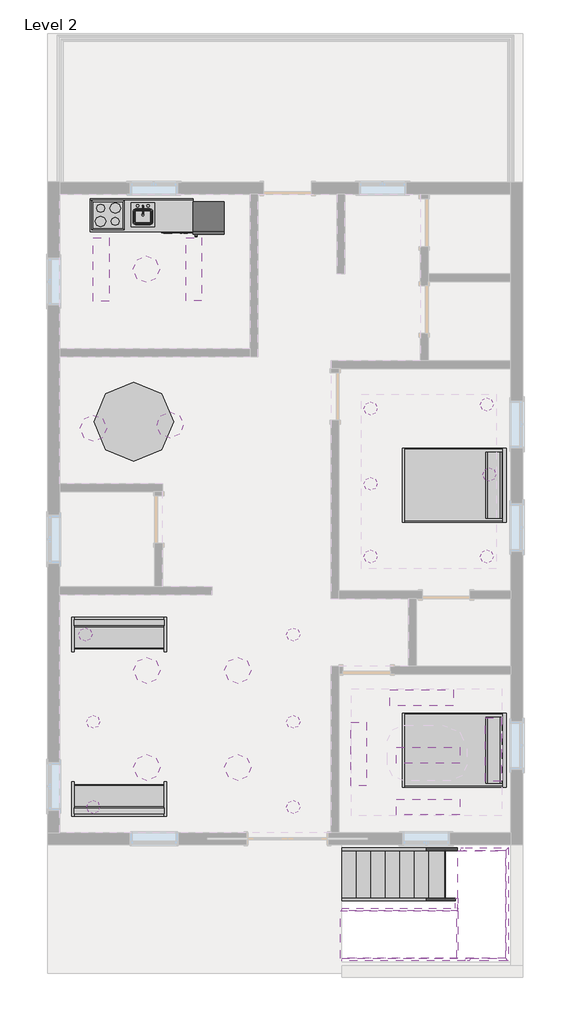
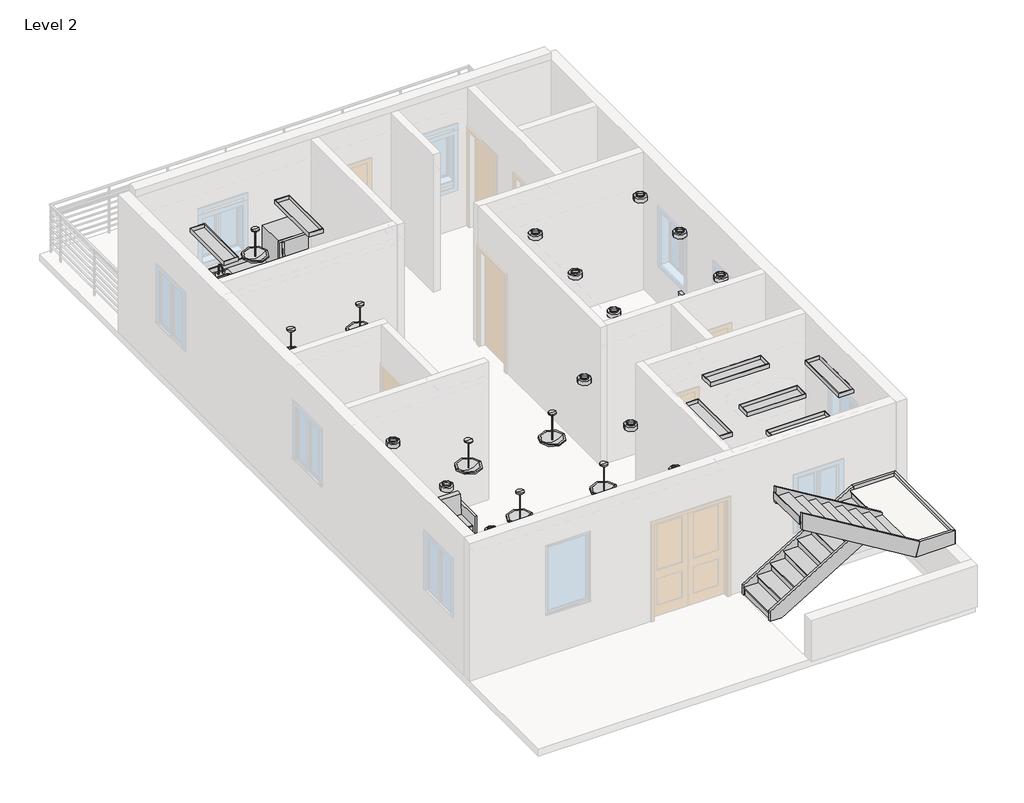
# One storey, part 3 of 3: 26 light fixtures, 8 members, 6 furniture elements, 4 proxies, 2 stair flights, 1 flow terminal, 1 slab.
"""IFC4 building model written with IfcOpenShell, lengths in millimetres."""

from ifc_helpers import new_model, si_unit, frame, origin, place, context, project, spatial, polyline, outline, extrude, faceted_brep, transform, mapped, element, save
from components import proxy_a6faaae8, proxy_45b28599, kitchenette_medium_kitchenette_medium_844211aa, proxy_c523a7b7, flow_terminal_871c2e40, furniture_096e7f55, furniture_c6510c7c, m_sofa_1830mm_f9e8a66b, furniture_bbcc68ce, ceiling_light_flat_round_60w_120v_0a96185f, ceiling_light_linear_box_1_x4_1_lamp_120v_8873ebfc, pendant_light_hemisphere_100w_120v_9c66a66f, non_monolithic_landing_dfce8634, stair_flight_5af034e0, stair_flight_d8780985

model = new_model("IFC4")

# Units and contexts
model_context = context("Model", 3, world=origin())
ifc_project = project(units=[si_unit("LENGTHUNIT", "METRE", prefix="MILLI")], contexts=[model_context])

# Site, building, storey
site = spatial("IfcSite", under=ifc_project)
building = spatial("IfcBuilding", under=site)
storey = spatial("IfcBuildingStorey", under=building, Name="Level 2", Elevation=3200.4)

# Proxies
placement = place(None, origin())
proxy_shape = proxy_a6faaae8(model_context)
element("IfcBuildingElementProxy", 1, Name="Cook Top-4 Unit2 : 22\" x 20\"", ObjectType="Cook Top-4 Unit2 : 22\" x 20\"", at=placement, inside=storey, context=model_context, shape_type="MappedRepresentation", body=[
    mapped(proxy_shape, transform((-8911.7572065, 13575.3206867, 3200.4), x_axis=(1.0, 0.0, 0.0), y_axis=(0.0, 1.0, 0.0), z_axis=(0.0, 0.0, 1.0))),
])
proxy_2_shape = proxy_45b28599(model_context)
element("IfcBuildingElementProxy", 2, Name="Dishwasher : 24\" x 24\" x 34\"", ObjectType="Dishwasher : 24\" x 24\" x 34\"", at=placement, inside=storey, context=model_context, shape_type="MappedRepresentation", body=[
    mapped(proxy_2_shape, transform((-7960.574675, 13283.4711219, 3200.4), x_axis=(1.0, 0.0, 0.0), y_axis=(0.0, 1.0, 0.0), z_axis=(0.0, 0.0, 1.0))),
])
kitchenette_medium_kitchenette_medium_shape = kitchenette_medium_kitchenette_medium_844211aa(model_context)
element("IfcBuildingElementProxy", 3, Name="Kitchenette - Medium : Kitchenette - Medium", ObjectType="Kitchenette - Medium : Kitchenette - Medium", at=placement, inside=storey, context=model_context, shape_type="MappedRepresentation", body=[
    mapped(kitchenette_medium_kitchenette_medium_shape, transform((-8587.5949114, 13880.1206867, 3200.4), x_axis=(1.0, 0.0, 0.0), y_axis=(0.0, 1.0, 0.0), z_axis=(0.0, 0.0, 1.0))),
])
proxy_3_shape = proxy_c523a7b7(model_context)
element("IfcBuildingElementProxy", 4, Name="Refrigerator : 24\" x 25\" LH", ObjectType="Refrigerator : 24\" x 25\" LH", at=placement, inside=storey, context=model_context, shape_type="MappedRepresentation", body=[
    mapped(proxy_3_shape, transform((-6975.0072065, 13529.6717152, 3200.4), x_axis=(1.0, 0.0, 0.0), y_axis=(0.0, 1.0, 0.0), z_axis=(0.0, 0.0, 1.0))),
])

# Flow terminal
flow_terminal_shape = flow_terminal_871c2e40(model_context)
element("IfcFlowTerminal", 5, ObjectType="Sink Kitchen-Island : 18\" x 18\"", at=placement, inside=storey, context=model_context, shape_type="MappedRepresentation", body=[
    mapped(flow_terminal_shape, transform((-8254.3464471, 13572.9752855, 3186.0), x_axis=(1.0, 0.0, 0.0), y_axis=(0.0, 1.0, 0.0), z_axis=(0.0, 0.0, 1.0))),
])

# Furniture
furniture_shape = furniture_096e7f55(model_context)
element("IfcFurniture", 6, ObjectType="Bed-Shaker : Double 56\" x 78\"", at=placement, inside=storey, context=model_context, shape_type="MappedRepresentation", body=[
    mapped(furniture_shape, transform((-1266.3572065, 8361.9706867, 3200.4), x_axis=(0.0, -1.0000000000000007, 0.0), y_axis=(1.0000000000000007, 0.0, 0.0), z_axis=(0.0, 0.0, 1.0))),
])
element("IfcFurniture", 7, ObjectType="Bed-Shaker : Double 56\" x 78\"", at=placement, inside=storey, context=model_context, shape_type="MappedRepresentation", body=[
    mapped(furniture_shape, transform((-1266.3572065, 3269.2706867, 3200.4), x_axis=(0.0, -1.0, 0.0), y_axis=(1.0, 0.0, 0.0), z_axis=(0.0, 0.0, 1.0))),
])
furniture_2_shape = furniture_c6510c7c(model_context)
element("IfcFurniture", 8, ObjectType="Counter Top w Sink Hole : 24\" Depth", at=placement, inside=storey, context=model_context, shape_type="MappedRepresentation", body=[
    mapped(furniture_2_shape, transform((-8054.1949114, 13880.1206867, 3186.0), x_axis=(1.0, 0.0, 0.0), y_axis=(0.0, 1.0, 0.0), z_axis=(0.0, 0.0, 1.0))),
])
m_sofa_1830mm_shape = m_sofa_1830mm_f9e8a66b(model_context)
element("IfcFurniture", 9, ObjectType="M_Sofa : 1830mm", at=placement, inside=storey, context=model_context, shape_type="MappedRepresentation", body=[
    mapped(m_sofa_1830mm_shape, transform((-8766.2276983, 5364.6665883, 3200.4), x_axis=(1.0, 0.0, 0.0), y_axis=(0.0, 1.0, 0.0), z_axis=(0.0, 0.0, 1.0))),
])
element("IfcFurniture", 10, ObjectType="M_Sofa : 1830mm", at=placement, inside=storey, context=model_context, shape_type="MappedRepresentation", body=[
    mapped(m_sofa_1830mm_shape, transform((-8625.4867147, 2494.674785, 3200.4), x_axis=(-1.0000000000000002, 0.0, 0.0), y_axis=(0.0, -1.0000000000000002, 0.0), z_axis=(0.0, 0.0, 1.0))),
])
furniture_3_shape = furniture_bbcc68ce(model_context)
element("IfcFurniture", 11, ObjectType="Table-Dining Round w Chairs : 60\" Diameter", at=placement, inside=storey, context=model_context, shape_type="MappedRepresentation", body=[
    mapped(furniture_3_shape, transform((-8517.0768878, 9782.3608189, 3200.4), x_axis=(1.0, 0.0, 0.0), y_axis=(0.0, 1.0, 0.0), z_axis=(0.0, 0.0, 1.0))),
])

# Light fixtures
ceiling_light_flat_round_60w_120v_shape = ceiling_light_flat_round_60w_120v_0a96185f(model_context)
element("IfcLightFixture", 12, ObjectType="Ceiling Light - Flat Round : 60W - 120V", at=placement, inside=storey, context=model_context, shape_type="MappedRepresentation", body=[
    mapped(ceiling_light_flat_round_60w_120v_shape, transform((-9343.5572065, 5510.8206867, 3403.6), x_axis=(1.0, 0.0, 0.0), y_axis=(0.0, 1.0, 0.0), z_axis=(0.0, 0.0, 1.0))),
])
element("IfcLightFixture", 13, ObjectType="Ceiling Light - Flat Round : 60W - 120V", at=placement, inside=storey, context=model_context, shape_type="MappedRepresentation", body=[
    mapped(ceiling_light_flat_round_60w_120v_shape, transform((-5345.2061474, 5507.5682565, 3403.6), x_axis=(1.0, 0.0, 0.0), y_axis=(0.0, 1.0, 0.0), z_axis=(0.0, 0.0, 1.0))),
])
element("IfcLightFixture", 14, ObjectType="Ceiling Light - Flat Round : 60W - 120V", at=placement, inside=storey, context=model_context, shape_type="MappedRepresentation", body=[
    mapped(ceiling_light_flat_round_60w_120v_shape, transform((-9193.3061474, 3831.1682565, 3403.6), x_axis=(1.0, 0.0, 0.0), y_axis=(0.0, 1.0, 0.0), z_axis=(0.0, 0.0, 1.0))),
])
element("IfcLightFixture", 15, ObjectType="Ceiling Light - Flat Round : 60W - 120V", at=placement, inside=storey, context=model_context, shape_type="MappedRepresentation", body=[
    mapped(ceiling_light_flat_round_60w_120v_shape, transform((-5345.2061474, 3831.1682565, 3403.6), x_axis=(1.0, 0.0, 0.0), y_axis=(0.0, 1.0, 0.0), z_axis=(0.0, 0.0, 1.0))),
])
element("IfcLightFixture", 16, ObjectType="Ceiling Light - Flat Round : 60W - 120V", at=placement, inside=storey, context=model_context, shape_type="MappedRepresentation", body=[
    mapped(ceiling_light_flat_round_60w_120v_shape, transform((-9193.3061474, 2192.8682565, 3403.6), x_axis=(1.0, 0.0, 0.0), y_axis=(0.0, 1.0, 0.0), z_axis=(0.0, 0.0, 1.0))),
])
element("IfcLightFixture", 17, ObjectType="Ceiling Light - Flat Round : 60W - 120V", at=placement, inside=storey, context=model_context, shape_type="MappedRepresentation", body=[
    mapped(ceiling_light_flat_round_60w_120v_shape, transform((-5345.2061474, 2192.8682565, 3403.6), x_axis=(1.0, 0.0, 0.0), y_axis=(0.0, 1.0, 0.0), z_axis=(0.0, 0.0, 1.0))),
])
element("IfcLightFixture", 18, ObjectType="Ceiling Light - Flat Round : 60W - 277V", at=placement, inside=storey, context=model_context, shape_type="MappedRepresentation", body=[
    mapped(ceiling_light_flat_round_60w_120v_shape, transform((-3860.0824155, 9852.6859166, 3454.4), x_axis=(1.0, 0.0, 0.0), y_axis=(0.0, 1.0, 0.0), z_axis=(0.0, 0.0, 1.0))),
])
element("IfcLightFixture", 19, ObjectType="Ceiling Light - Flat Round : 60W - 277V", at=placement, inside=storey, context=model_context, shape_type="MappedRepresentation", body=[
    mapped(ceiling_light_flat_round_60w_120v_shape, transform((-1624.8824155, 9928.8859166, 3454.4), x_axis=(1.0, 0.0, 0.0), y_axis=(0.0, 1.0, 0.0), z_axis=(0.0, 0.0, 1.0))),
])
element("IfcLightFixture", 20, ObjectType="Ceiling Light - Flat Round : 60W - 277V", at=placement, inside=storey, context=model_context, shape_type="MappedRepresentation", body=[
    mapped(ceiling_light_flat_round_60w_120v_shape, transform((-1574.0824155, 8582.6859166, 3454.4), x_axis=(1.0, 0.0, 0.0), y_axis=(0.0, 1.0, 0.0), z_axis=(0.0, 0.0, 1.0))),
])
element("IfcLightFixture", 21, ObjectType="Ceiling Light - Flat Round : 60W - 277V", at=placement, inside=storey, context=model_context, shape_type="MappedRepresentation", body=[
    mapped(ceiling_light_flat_round_60w_120v_shape, transform((-3860.0824155, 8404.8859166, 3454.4), x_axis=(1.0, 0.0, 0.0), y_axis=(0.0, 1.0, 0.0), z_axis=(0.0, 0.0, 1.0))),
])
element("IfcLightFixture", 22, ObjectType="Ceiling Light - Flat Round : 60W - 277V", at=placement, inside=storey, context=model_context, shape_type="MappedRepresentation", body=[
    mapped(ceiling_light_flat_round_60w_120v_shape, transform((-3860.0824155, 7007.8859166, 3454.4), x_axis=(1.0, 0.0, 0.0), y_axis=(0.0, 1.0, 0.0), z_axis=(0.0, 0.0, 1.0))),
])
element("IfcLightFixture", 23, ObjectType="Ceiling Light - Flat Round : 60W - 277V", at=placement, inside=storey, context=model_context, shape_type="MappedRepresentation", body=[
    mapped(ceiling_light_flat_round_60w_120v_shape, transform((-1624.8824155, 7007.8859166, 3454.4), x_axis=(1.0, 0.0, 0.0), y_axis=(0.0, 1.0, 0.0), z_axis=(0.0, 0.0, 1.0))),
])
ceiling_light_linear_box_1_x4_1_lamp_120v_shape = ceiling_light_linear_box_1_x4_1_lamp_120v_8873ebfc(model_context)
element("IfcLightFixture", 24, ObjectType="Ceiling Light - Linear Box : 1'x4'(1 Lamp) - 120V", at=placement, inside=storey, context=model_context, shape_type="MappedRepresentation", body=[
    mapped(ceiling_light_linear_box_1_x4_1_lamp_120v_shape, transform((-9038.7572065, 12521.2206867, 3403.6), x_axis=(0.0, 1.0000000000000002, 0.0), y_axis=(-1.0000000000000002, 0.0, 0.0), z_axis=(0.0, 0.0, 1.0))),
])
element("IfcLightFixture", 25, ObjectType="Ceiling Light - Linear Box : 1'x4'(1 Lamp) - 120V", at=placement, inside=storey, context=model_context, shape_type="MappedRepresentation", body=[
    mapped(ceiling_light_linear_box_1_x4_1_lamp_120v_shape, transform((-7259.0575781, 12529.2390316, 3403.6), x_axis=(0.0, -1.0000000000000007, 0.0), y_axis=(1.0000000000000007, 0.0, 0.0), z_axis=(0.0, 0.0, 1.0))),
])
element("IfcLightFixture", 26, ObjectType="Ceiling Light - Linear Box : 1'x4'(2 Lamp) - 120V", at=placement, inside=storey, context=model_context, shape_type="MappedRepresentation", body=[
    mapped(ceiling_light_linear_box_1_x4_1_lamp_120v_shape, transform((-2753.8070542, 3185.9258823, 3403.6), x_axis=(1.0, 0.0, 0.0), y_axis=(0.0, 1.0, 0.0), z_axis=(0.0, 0.0, 1.0))),
])
element("IfcLightFixture", 27, ObjectType="Ceiling Light - Linear Box : 1'x4'(2 Lamp) - 120V", at=placement, inside=storey, context=model_context, shape_type="MappedRepresentation", body=[
    mapped(ceiling_light_linear_box_1_x4_1_lamp_120v_shape, transform((-2880.8070542, 4290.8258823, 3441.6205268), x_axis=(1.0, 0.0, 0.0), y_axis=(0.0, 1.0, 0.0), z_axis=(0.0, 0.0, 1.0))),
])
element("IfcLightFixture", 28, ObjectType="Ceiling Light - Linear Box : 1'x4'(2 Lamp) - 120V", at=placement, inside=storey, context=model_context, shape_type="MappedRepresentation", body=[
    mapped(ceiling_light_linear_box_1_x4_1_lamp_120v_shape, transform((-2753.8070542, 2195.3258823, 3441.6205268), x_axis=(1.0, 0.0, 0.0), y_axis=(0.0, 1.0, 0.0), z_axis=(0.0, 0.0, 1.0))),
])
element("IfcLightFixture", 29, ObjectType="Ceiling Light - Linear Box : 1'x4'(2 Lamp) - 120V", at=placement, inside=storey, context=model_context, shape_type="MappedRepresentation", body=[
    mapped(ceiling_light_linear_box_1_x4_1_lamp_120v_shape, transform((-1496.5070542, 3300.2258823, 3441.6205268), x_axis=(0.0, 1.0000000000000002, 0.0), y_axis=(-1.0000000000000002, 0.0, 0.0), z_axis=(0.0, 0.0, 1.0))),
])
element("IfcLightFixture", 30, ObjectType="Ceiling Light - Linear Box : 1'x4'(2 Lamp) - 120V", at=placement, inside=storey, context=model_context, shape_type="MappedRepresentation", body=[
    mapped(ceiling_light_linear_box_1_x4_1_lamp_120v_shape, transform((-4087.3070542, 3211.3258823, 3441.6205268), x_axis=(0.0, 1.0000000000000002, 0.0), y_axis=(-1.0000000000000002, 0.0, 0.0), z_axis=(0.0, 0.0, 1.0))),
])
pendant_light_hemisphere_100w_120v_shape = pendant_light_hemisphere_100w_120v_9c66a66f(model_context)
element("IfcLightFixture", 31, ObjectType="Pendant Light - Hemisphere : 100W - 120V", at=placement, inside=storey, context=model_context, shape_type="MappedRepresentation", body=[
    mapped(pendant_light_hemisphere_100w_120v_shape, transform((-8164.6061474, 2954.8682565, 3403.6), x_axis=(1.0, 0.0, 0.0), y_axis=(0.0, 1.0, 0.0), z_axis=(0.0, 0.0, 1.0))),
])
element("IfcLightFixture", 32, ObjectType="Pendant Light - Hemisphere : 100W - 120V", at=placement, inside=storey, context=model_context, shape_type="MappedRepresentation", body=[
    mapped(pendant_light_hemisphere_100w_120v_shape, transform((-8164.6061474, 4821.7682565, 3403.6), x_axis=(1.0, 0.0, 0.0), y_axis=(0.0, 1.0, 0.0), z_axis=(0.0, 0.0, 1.0))),
])
element("IfcLightFixture", 33, ObjectType="Pendant Light - Hemisphere : 100W - 120V", at=placement, inside=storey, context=model_context, shape_type="MappedRepresentation", body=[
    mapped(pendant_light_hemisphere_100w_120v_shape, transform((-6412.0061474, 4821.7682565, 3403.6), x_axis=(1.0, 0.0, 0.0), y_axis=(0.0, 1.0, 0.0), z_axis=(0.0, 0.0, 1.0))),
])
element("IfcLightFixture", 34, ObjectType="Pendant Light - Hemisphere : 100W - 120V", at=placement, inside=storey, context=model_context, shape_type="MappedRepresentation", body=[
    mapped(pendant_light_hemisphere_100w_120v_shape, transform((-6412.0061474, 2954.8682565, 3403.6), x_axis=(1.0, 0.0, 0.0), y_axis=(0.0, 1.0, 0.0), z_axis=(0.0, 0.0, 1.0))),
])
element("IfcLightFixture", 35, ObjectType="Pendant Light - Hemisphere : 100W - 120V", at=placement, inside=storey, context=model_context, shape_type="MappedRepresentation", body=[
    mapped(pendant_light_hemisphere_100w_120v_shape, transform((-9191.1572065, 9473.2206867, 3403.6), x_axis=(1.0, 0.0, 0.0), y_axis=(0.0, 1.0, 0.0), z_axis=(0.0, 0.0, 1.0))),
])
element("IfcLightFixture", 36, ObjectType="Pendant Light - Hemisphere : 100W - 120V", at=placement, inside=storey, context=model_context, shape_type="MappedRepresentation", body=[
    mapped(pendant_light_hemisphere_100w_120v_shape, transform((-7715.9326808, 9533.782557, 3403.6), x_axis=(1.0, 0.0, 0.0), y_axis=(0.0, 1.0, 0.0), z_axis=(0.0, 0.0, 1.0))),
])
element("IfcLightFixture", 37, ObjectType="Pendant Light - Hemisphere : 100W - 120V", at=placement, inside=storey, context=model_context, shape_type="MappedRepresentation", body=[
    mapped(pendant_light_hemisphere_100w_120v_shape, transform((-8173.4575781, 12529.2390316, 3403.6), x_axis=(1.0, 0.0, 0.0), y_axis=(0.0, 1.0, 0.0), z_axis=(0.0, 0.0, 1.0))),
])

# Members
element("IfcMember", 38, ObjectType="Stringer - 2\" Width", at=placement, inside=storey, context=model_context, shape_type="SweptSolid", body=[
    extrude(outline(polyline([(3412.514512, -4412.1017807), (3200.4, -4412.1017807), (3200.4, -4174.0162689), (4495.8, -2036.6062689), (4800.6, -2121.7607254), (3412.514512, -4412.1017807)])), frame((0.0, 1358.5428136, 0.0), z_axis=(0.0, 1.0, 0.0), x_axis=(0.0, 0.0, 1.0)), (0.0, 0.0, 1.0), 50.8),
])
element("IfcMember", 39, ObjectType="Stringer - 2\" Width", at=placement, inside=storey, context=model_context, shape_type="SweptSolid", body=[
    extrude(outline(polyline([(3412.514512, -4412.1017807), (3200.4, -4412.1017807), (3200.4, -4174.0162689), (4379.9845383, -2227.7017807), (4736.3932998, -2227.7017807), (3412.514512, -4412.1017807)])), frame((0.0, 393.3428136, 0.0), z_axis=(0.0, 1.0, 0.0), x_axis=(0.0, 0.0, 1.0)), (0.0, 0.0, 1.0), 50.8),
])
element("IfcMember", 40, ObjectType="Stringer - 2\" Width", at=placement, inside=storey, context=model_context, shape_type="SweptSolid", body=[
    extrude(outline(polyline([(4495.8, -2037.7972924), (4800.6, -1952.6428359), (6291.1811786, -4412.1017807), (5934.7724171, -4412.1017807), (4495.8, -2037.7972924)])), frame((0.0, -762.9793133, 0.0), z_axis=(0.0, 1.0, 0.0), x_axis=(0.0, 0.0, 1.0)), (0.0, 0.0, 1.0), 50.8),
])
element("IfcMember", 41, ObjectType="Stringer - 2\" Width", at=placement, inside=storey, context=model_context, shape_type="SweptSolid", body=[
    extrude(outline(polyline([(4580.1057504, -2176.9017807), (4936.514512, -2176.9017807), (6291.1811786, -4412.1017807), (5934.7724171, -4412.1017807), (4580.1057504, -2176.9017807)])), frame((0.0, 202.2206867, 0.0), z_axis=(0.0, 1.0, 0.0), x_axis=(0.0, 0.0, 1.0)), (0.0, 0.0, 1.0), 50.8),
])
element("IfcMember", 42, ObjectType="Stringer - 2\" Width", at=placement, inside=storey, context=model_context, shape_type="Brep", body=[
    faceted_brep([(-1952.6428359, -712.1793133, 4800.6), (-1952.6428359, -762.9793133, 4800.6), (-1211.7017807, -762.9793133, 4800.6), (-1262.5017807, -712.1793133, 4800.6), (-2037.7972924, -712.1793133, 4495.8), (-1262.5017807, -712.1793133, 4495.8), (-2037.7972924, -762.9793133, 4495.8), (-1211.7017807, -762.9793133, 4495.8)], [[[0, 1, 2, 3]], [[4, 0, 3, 5]], [[6, 4, 5, 7]], [[1, 6, 7, 2]], [[1, 0, 4, 6]], [[2, 7, 5, 3]]]),
])
element("IfcMember", 43, ObjectType="Stringer - 2\" Width", at=placement, inside=storey, context=model_context, shape_type="SweptSolid", body=[
    extrude(outline(polyline([(-1211.7017807, -762.9793133), (-1262.5017807, -712.1793133), (-1262.5017807, 1358.5428136), (-1211.7017807, 1409.3428136), (-1211.7017807, -762.9793133)])), frame((0.0, 0.0, 4495.8), z_axis=(0.0, 0.0, 1.0), x_axis=(1.0, 0.0, 0.0)), (0.0, 0.0, 1.0), 304.8),
])
element("IfcMember", 44, ObjectType="Stringer - 2\" Width", at=placement, inside=storey, context=model_context, shape_type="Brep", body=[
    faceted_brep([(-1262.5017807, 1358.5428136, 4800.6), (-1211.7017807, 1409.3428136, 4800.6), (-2121.7607254, 1409.3428136, 4800.6), (-2121.7607254, 1358.5428136, 4800.6), (-1262.5017807, 1358.5428136, 4495.8), (-2036.6062689, 1358.5428136, 4495.8), (-1211.7017807, 1409.3428136, 4495.8), (-2036.6062689, 1409.3428136, 4495.8)], [[[0, 1, 2, 3]], [[4, 0, 3, 5]], [[6, 4, 5, 7]], [[1, 6, 7, 2]], [[1, 0, 4, 6]], [[2, 7, 5, 3]]]),
])
element("IfcMember", 45, ObjectType="Stringer - 2\" Width", at=placement, inside=storey, context=model_context, shape_type="SweptSolid", body=[
    extrude(outline(polyline([(-2227.7017807, 444.1428136), (-2176.9017807, 444.1428136), (-2176.9017807, 253.0206867), (-2227.7017807, 253.0206867), (-2227.7017807, 444.1428136)])), frame((0.0, 0.0, 4495.8), z_axis=(0.0, 0.0, 1.0), x_axis=(1.0, 0.0, 0.0)), (0.0, 0.0, 1.0), 304.8),
])

# Slab
non_monolithic_landing_shape = non_monolithic_landing_dfce8634(model_context)
element("IfcSlab", 46, ObjectType="Non-Monolithic Landing", at=placement, inside=storey, context=model_context, shape_type="MappedRepresentation", body=[
    mapped(non_monolithic_landing_shape, transform((0.0, 0.0, 0.0), x_axis=(1.0, 0.0, 0.0), y_axis=(0.0, 1.0, 0.0), z_axis=(0.0, 0.0, 1.0))),
])

# Stair flights
stair_flight_shape = stair_flight_5af034e0(model_context)
element("IfcStairFlight", 47, ObjectType="2\" Tread 1\" Nosing 1/4\" Riser", at=placement, inside=storey, context=model_context, shape_type="MappedRepresentation", body=[
    mapped(stair_flight_shape, transform((0.0, 0.0, 0.0), x_axis=(1.0, 0.0, 0.0), y_axis=(0.0, 1.0, 0.0), z_axis=(0.0, 0.0, 1.0))),
])
stair_flight_2_shape = stair_flight_d8780985(model_context)
element("IfcStairFlight", 48, ObjectType="2\" Tread 1\" Nosing 1/4\" Riser", at=placement, inside=storey, context=model_context, shape_type="MappedRepresentation", body=[
    mapped(stair_flight_2_shape, transform((0.0, 0.0, 0.0), x_axis=(1.0, 0.0, 0.0), y_axis=(0.0, 1.0, 0.0), z_axis=(0.0, 0.0, 1.0))),
])

save(model, "model.ifc")

# Revit data of these elements
# Type "Cook Top-4 Unit2 : 22\" x 20\""
#   Depth = 1' - 8"
#   Width = 1' - 10"
#   Burner Material = Steel, Chrome Plated
#   Cooktop Material = Steel, Polished
#   Default Elevation = 0
#   Assembly Code = ""
# Type "Dishwasher : 24\" x 24\" x 34\""
#   Label = "DW"
#   Assembly Code = "E1090400"
#   Depth = 2' - 0"
#   Height = 2' - 10"
#   Width = 2' - 0"
#   Dishwasher Material = Steel, Paint Finish, Ivory, Glossy
#   Panel Face Material = Plastic, Opaque Black
#   Default Elevation = 0
# Type "Kitchenette - Medium : Kitchenette - Medium"
#   Assembly Code = "E1090400"
#   Counter Length = 6' - 6"
#   Cabinet Width = 4' - 6"
#   Cabinet Height = 2' - 10 1/2"
#   Cabinet Depth = 2' - 0"
#   Toe Depth = 0' - 3"
#   Toe Height = 0' - 3 1/2"
#   Cabinet Material = Cabinets
#   Door/Drawer Material = Cabinets
#   Handle Material = Cabinets - Handles
#   Default Elevation = 0
# Type "Refrigerator : 24\" x 25\" LH"
#   Label = "REF."
#   Assembly Code = "E1090400"
#   Depth = 2' - 0 3/4"
#   Handle = 0' - 1 1/2"
#   Height = 5' - 3 1/2"
#   Rear Clearance = 0' - 2"
#   Top Door Height = 1' - 8"
#   Width = 1' - 11 1/2"
#   Material = Steel, Paint Finish, Ivory, Glossy
#   Default Elevation = 0
# Type "Sink Kitchen-Island : 18\" x 18\""
#   Assembly Code = "D2010410"
#   Counter Height = 3' - 0"
#   Depth = 1' - 6"
#   Width = 1' - 6"
#   Faucet Material = Steel, Polished
#   Sink Material = Steel, Polished
#   Default Elevation = 0
# Type "Bed-Shaker : Double 56\" x 78\""
#   Assembly Code = "E2020200"
#   Length = 6' - 6"
#   Width = 4' - 8"
#   Frame Material = Birch
#   Mattress Material = Linen, White
#   Default Elevation = 0
# Type "Counter Top w Sink Hole : 24\" Depth"
#   Assembly Code = "C1030400"
#   Counter Thickness = 0' - 1 1/2"
#   Depth = 2' - 1"
#   Height = 3' - 0"
#   Length [instance default] = 8' - 0"
#   Sink Location [instance default] = 2' - 0"
#   Sink Location To Wall [instance default] = 0' - 6"
#   Sink Opening Depth [instance default] = 1' - 3"
#   Sink Opening Width [instance default] = 2' - 3"
#   Counter Top Material = none
#   Default Elevation = 0
# Type "M_Sofa : 1830mm"
#   Width = 6' - 0.04724"
#   Seat Material = Linen, Beige
#   Frame Material = Cherry
#   Default Elevation = 0
# Type "Table-Dining Round w Chairs : 60\" Diameter"
#   Assembly Code = "E2020200"
#   Radius = 2' - 6"
#   Diameter = 5' - 0"
#   Height = 2' - 6"
#   Chairs = 6
#   Base Material = Pine
#   Top Material = Laminate, Linen, Matte
#   Default Elevation = 0
# Type "Ceiling Light - Flat Round : 60W - 120V"
#   Lamp = "A-19"
#   Assembly Code = "D5020220"
#   Wattage = 60 W
#   built-in parameter 1150110 = 1 (stored number, unit not read)
#   built-in parameter 1114217 = 1 (stored number, unit not read)
#   built-in parameter 1150109 = 1 (stored number, unit not read)
#   built-in parameter 1150113 = 1 (stored number, unit not read)
#   built-in parameter 1150115 = 1 (stored number, unit not read)
#   built-in parameter 1150105 = 272.155 (stored number, unit not read)
#   Light Source Symbol Size = 2' - 0"
#   built-in parameter 1150112 = 1 (stored number, unit not read)
#   built-in parameter 1150114 = 1 (stored number, unit not read)
#   built-in parameter 1150107 = 2800 (stored number, unit not read)
#   built-in parameter 1150106 = 2.72155 (stored number, unit not read)
#   Emit from Circle Diameter = 0' - 10"
#   built-in parameter 1150104 = 1.32387 (stored number, unit not read)
#   Ballast Voltage = 120 V
#   built-in parameter 1114218 = 1 (stored number, unit not read)
#   built-in parameter 1150133 = 10 (stored number, unit not read)
#   Lumens = 855 lm
#   Apparent Load = 60 VA
#   built-in parameter 1150134 = 4
#   built-in parameter 1150137 = 1
#   Color Filter = 16777215
#   built-in parameter 1140040 [instance default] = 1
#   Ballast Number of Poles = 1
#   Light Box Material = Steel, Paint Finish, Dark Gray, Matte
#   Diffuser Material = Glass, White, High Luminance
#   Wattage Comments = ""
#   Emit Shape Visible in Rendering = no
#   Dimming Lamp Color Temperature Shift = (empty or 0)
#   Default Elevation = 0
# Type "Ceiling Light - Flat Round : 60W - 277V"
#   Lamp = "A-19"
#   Assembly Code = "D5020220"
#   Wattage = 60 W
#   built-in parameter 1150110 = 1 (stored number, unit not read)
#   built-in parameter 1114217 = 1 (stored number, unit not read)
#   built-in parameter 1150109 = 1 (stored number, unit not read)
#   built-in parameter 1150113 = 1 (stored number, unit not read)
#   built-in parameter 1150115 = 1 (stored number, unit not read)
#   built-in parameter 1150105 = 272.155 (stored number, unit not read)
#   Light Source Symbol Size = 2' - 0"
#   built-in parameter 1150112 = 1 (stored number, unit not read)
#   built-in parameter 1150114 = 1 (stored number, unit not read)
#   built-in parameter 1150107 = 2800 (stored number, unit not read)
#   built-in parameter 1150106 = 2.72155 (stored number, unit not read)
#   Emit from Circle Diameter = 0' - 10"
#   built-in parameter 1150104 = 1.32387 (stored number, unit not read)
#   Ballast Voltage = 277 V
#   built-in parameter 1114218 = 1 (stored number, unit not read)
#   built-in parameter 1150133 = 10 (stored number, unit not read)
#   Lumens = 855 lm
#   Apparent Load = 60 VA
#   built-in parameter 1150134 = 4
#   built-in parameter 1150137 = 1
#   Color Filter = 16777215
#   built-in parameter 1140040 [instance default] = 1
#   Ballast Number of Poles = 1
#   Light Box Material = Steel, Paint Finish, Dark Gray, Matte
#   Diffuser Material = Glass, White, High Luminance
#   Wattage Comments = ""
#   Emit Shape Visible in Rendering = no
#   Dimming Lamp Color Temperature Shift = (empty or 0)
#   Default Elevation = 0
# Type "Ceiling Light - Linear Box : 1'x4'(1 Lamp) - 120V"
#   Assembly Code = "D5020210"
#   Lamp = "T-12"
#   Wattage = 40 W
#   built-in parameter 1150110 = 1 (stored number, unit not read)
#   built-in parameter 1114217 = 0.88 (stored number, unit not read)
#   built-in parameter 1150109 = 1 (stored number, unit not read)
#   built-in parameter 1150113 = 1 (stored number, unit not read)
#   built-in parameter 1150115 = 1 (stored number, unit not read)
#   built-in parameter 1150105 = 1002.68 (stored number, unit not read)
#   Light Source Symbol Size = 2' - 0"
#   built-in parameter 1150112 = 1 (stored number, unit not read)
#   built-in parameter 1150114 = 1 (stored number, unit not read)
#   built-in parameter 1150107 = 4230 (stored number, unit not read)
#   built-in parameter 1150106 = 10.0268 (stored number, unit not read)
#   Emit from Rectangle Width = 0' - 11"
#   Emit from Rectangle Length = 3' - 11"
#   built-in parameter 1150104 = 7.31611 (stored number, unit not read)
#   Ballast Voltage = 120 V
#   built-in parameter 1114218 = 0.88 (stored number, unit not read)
#   built-in parameter 1150133 = 10 (stored number, unit not read)
#   Box Length = 4' - 0"
#   Lumens = 3150 lm
#   Box Width = 1' - 0"
#   Apparent Load = 40 VA
#   built-in parameter 1150134 = 8
#   built-in parameter 1150137 = 1
#   Color Filter = 16777215
#   Ballast Number of Poles = 1
#   Diffuser Material = Glass, White, High Luminance
#   Light Box Material = Steel, Paint Finish, Ivory, Glossy
#   Emit Shape Visible in Rendering = no
#   Dimming Lamp Color Temperature Shift = (empty or 0)
#   Default Elevation = 0
# Type "Ceiling Light - Linear Box : 1'x4'(2 Lamp) - 120V"
#   Assembly Code = "D5020210"
#   Lamp = "T-12"
#   Wattage = 80 W
#   built-in parameter 1150110 = 1 (stored number, unit not read)
#   built-in parameter 1114217 = 0.88 (stored number, unit not read)
#   built-in parameter 1150109 = 1 (stored number, unit not read)
#   built-in parameter 1150113 = 1 (stored number, unit not read)
#   built-in parameter 1150115 = 1 (stored number, unit not read)
#   built-in parameter 1150105 = 2005.35 (stored number, unit not read)
#   Light Source Symbol Size = 2' - 0"
#   built-in parameter 1150112 = 1 (stored number, unit not read)
#   built-in parameter 1150114 = 1 (stored number, unit not read)
#   built-in parameter 1150107 = 4230 (stored number, unit not read)
#   built-in parameter 1150106 = 20.0535 (stored number, unit not read)
#   Emit from Rectangle Width = 0' - 11"
#   Emit from Rectangle Length = 3' - 11"
#   built-in parameter 1150104 = 7.31611 (stored number, unit not read)
#   Ballast Voltage = 120 V
#   built-in parameter 1114218 = 0.88 (stored number, unit not read)
#   built-in parameter 1150133 = 10 (stored number, unit not read)
#   Box Length = 4' - 0"
#   Lumens = 6300 lm
#   Box Width = 1' - 0"
#   Apparent Load = 80 VA
#   built-in parameter 1150134 = 8
#   built-in parameter 1150137 = 1
#   Color Filter = 16777215
#   Ballast Number of Poles = 1
#   Diffuser Material = Glass, White, High Luminance
#   Light Box Material = Steel, Paint Finish, Ivory, Glossy
#   Emit Shape Visible in Rendering = no
#   Dimming Lamp Color Temperature Shift = (empty or 0)
#   Default Elevation = 0
# Type "Pendant Light - Hemisphere : 100W - 120V"
#   Lamp = "A-19"
#   Assembly Code = "D5020220"
#   Wattage = 100 W
#   built-in parameter 1150110 = 1 (stored number, unit not read)
#   built-in parameter 1114217 = 1 (stored number, unit not read)
#   built-in parameter 1150109 = 1 (stored number, unit not read)
#   built-in parameter 1150113 = 1 (stored number, unit not read)
#   built-in parameter 1150115 = 1 (stored number, unit not read)
#   built-in parameter 1150105 = 537.944 (stored number, unit not read)
#   Light Source Symbol Size = 2' - 0"
#   built-in parameter 1150112 = 1 (stored number, unit not read)
#   built-in parameter 1150114 = 1 (stored number, unit not read)
#   built-in parameter 1150107 = 2800 (stored number, unit not read)
#   built-in parameter 1150106 = 5.37944 (stored number, unit not read)
#   built-in parameter 1150104 = 1.57006 (stored number, unit not read)
#   Ballast Voltage = 120 V
#   built-in parameter 1114218 = 1 (stored number, unit not read)
#   built-in parameter 1150133 = 10 (stored number, unit not read)
#   Drop From Ceiling = 2' - 3"
#   Lumens = 1690 lm
#   Apparent Load = 100 VA
#   built-in parameter 1150134 = 4
#   built-in parameter 1150137 = 1
#   Color Filter = 16777215
#   built-in parameter 1140040 [instance default] = 1
#   Ballast Number of Poles = 1
#   Ceiling Mount Material = Steel, Chrome Plated
#   Pendant Material = Glass, Frosted
#   Dimming Lamp Color Temperature Shift = (empty or 0)
#   Default Elevation = 0
#   Wattage Comments = ""
# Element 1 (IfcBuildingElementProxy, "Cook Top-4 Unit2 : 22\" x 20\"")
#   Phase Created = New Construction
#   Materials on its faces: "Steel, Chrome Plated", "Steel, Polished"
# Element 2 (IfcBuildingElementProxy, "Dishwasher : 24\" x 24\" x 34\"")
#   Phase Created = New Construction
#   Materials on its faces: "Steel, Paint Finish, Ivory, Glossy", "Plastic, Opaque Black"
# Element 3 (IfcBuildingElementProxy, "Kitchenette - Medium : Kitchenette - Medium")
#   Phase Created = New Construction
#   Materials on its faces: "Cabinets", "Cabinets - Handles"
# Element 4 (IfcBuildingElementProxy, "Refrigerator : 24\" x 25\" LH")
#   Phase Created = New Construction
#   Materials on its faces: "Steel, Paint Finish, Ivory, Glossy", "Steel, Chrome Plated"
# Element 5 (IfcFlowTerminal, "Sink Kitchen-Island : 18\" x 18\"")
#   Mark = "6"
#   Phase Created = New Construction
#   Materials on its faces: "Steel, Polished"
# Elements 6, 7 (IfcFurniture, "Bed-Shaker : Double 56\" x 78\"")
#   Phase Created = New Construction
#   Materials on its faces: "Birch", "Linen, White"
# Element 8 (IfcFurniture, "Counter Top w Sink Hole : 24\" Depth")
#   Sink Opening Depth = 1' - 2"
#   Sink Location To Wall = 0' - 6"
#   Length = 6' - 6"
#   Sink Location = 3' - 4"
#   Sink Opening Width = 1' - 4"
#   Phase Created = New Construction
#   Materials on its faces: "Counter Top"
# Elements 9, 10 (IfcFurniture, "M_Sofa : 1830mm")
#   Phase Created = New Construction
#   Materials on its faces: "Cherry", "Linen, Beige"
# Element 11 (IfcFurniture, "Table-Dining Round w Chairs : 60\" Diameter")
#   Phase Created = New Construction
#   Materials on its faces: "Pine", "Laminate, Linen, Matte"
# Element 12 (IfcLightFixture, "Ceiling Light - Flat Round : 60W - 120V")
#   Mark = "43"
#   built-in parameter 1140040 = 1
#   Phase Created = New Construction
#   Materials on its faces: "Glass, White, High Luminance", "Steel, Paint Finish, Dark Gray, Matte"
# Element 13 (IfcLightFixture, "Ceiling Light - Flat Round : 60W - 120V")
#   Mark = "44"
#   built-in parameter 1140040 = 1
#   Phase Created = New Construction
#   Materials on its faces: "Glass, White, High Luminance", "Steel, Paint Finish, Dark Gray, Matte"
# Element 14 (IfcLightFixture, "Ceiling Light - Flat Round : 60W - 120V")
#   Mark = "45"
#   built-in parameter 1140040 = 1
#   Phase Created = New Construction
#   Materials on its faces: "Glass, White, High Luminance", "Steel, Paint Finish, Dark Gray, Matte"
# Element 15 (IfcLightFixture, "Ceiling Light - Flat Round : 60W - 120V")
#   Mark = "46"
#   built-in parameter 1140040 = 1
#   Phase Created = New Construction
#   Materials on its faces: "Glass, White, High Luminance", "Steel, Paint Finish, Dark Gray, Matte"
# Element 16 (IfcLightFixture, "Ceiling Light - Flat Round : 60W - 120V")
#   Mark = "47"
#   built-in parameter 1140040 = 1
#   Phase Created = New Construction
#   Materials on its faces: "Glass, White, High Luminance", "Steel, Paint Finish, Dark Gray, Matte"
# Element 17 (IfcLightFixture, "Ceiling Light - Flat Round : 60W - 120V")
#   Mark = "48"
#   built-in parameter 1140040 = 1
#   Phase Created = New Construction
#   Materials on its faces: "Glass, White, High Luminance", "Steel, Paint Finish, Dark Gray, Matte"
# Element 18 (IfcLightFixture, "Ceiling Light - Flat Round : 60W - 277V")
#   Mark = "27"
#   built-in parameter 1140040 = 1
#   Phase Created = New Construction
#   Materials on its faces: "Glass, White, High Luminance", "Steel, Paint Finish, Dark Gray, Matte"
# Element 19 (IfcLightFixture, "Ceiling Light - Flat Round : 60W - 277V")
#   Mark = "28"
#   built-in parameter 1140040 = 1
#   Phase Created = New Construction
#   Materials on its faces: "Glass, White, High Luminance", "Steel, Paint Finish, Dark Gray, Matte"
# Element 20 (IfcLightFixture, "Ceiling Light - Flat Round : 60W - 277V")
#   Mark = "29"
#   built-in parameter 1140040 = 1
#   Phase Created = New Construction
#   Materials on its faces: "Glass, White, High Luminance", "Steel, Paint Finish, Dark Gray, Matte"
# Element 21 (IfcLightFixture, "Ceiling Light - Flat Round : 60W - 277V")
#   Mark = "30"
#   built-in parameter 1140040 = 1
#   Phase Created = New Construction
#   Materials on its faces: "Glass, White, High Luminance", "Steel, Paint Finish, Dark Gray, Matte"
# Element 22 (IfcLightFixture, "Ceiling Light - Flat Round : 60W - 277V")
#   Mark = "31"
#   built-in parameter 1140040 = 1
#   Phase Created = New Construction
#   Materials on its faces: "Glass, White, High Luminance", "Steel, Paint Finish, Dark Gray, Matte"
# Element 23 (IfcLightFixture, "Ceiling Light - Flat Round : 60W - 277V")
#   Mark = "32"
#   built-in parameter 1140040 = 1
#   Phase Created = New Construction
#   Materials on its faces: "Glass, White, High Luminance", "Steel, Paint Finish, Dark Gray, Matte"
# Element 24 (IfcLightFixture, "Ceiling Light - Linear Box : 1'x4'(1 Lamp) - 120V")
#   Mark = "55"
#   Phase Created = New Construction
#   Materials on its faces: "Steel, Paint Finish, Ivory, Glossy", "Glass, White, High Luminance"
# Element 25 (IfcLightFixture, "Ceiling Light - Linear Box : 1'x4'(1 Lamp) - 120V")
#   Mark = "56"
#   Phase Created = New Construction
#   Materials on its faces: "Steel, Paint Finish, Ivory, Glossy", "Glass, White, High Luminance"
# Element 26 (IfcLightFixture, "Ceiling Light - Linear Box : 1'x4'(2 Lamp) - 120V")
#   Mark = "38"
#   Phase Created = New Construction
#   Materials on its faces: "Steel, Paint Finish, Ivory, Glossy", "Glass, White, High Luminance"
# Element 27 (IfcLightFixture, "Ceiling Light - Linear Box : 1'x4'(2 Lamp) - 120V")
#   Mark = "39"
#   Phase Created = New Construction
#   Materials on its faces: "Steel, Paint Finish, Ivory, Glossy", "Glass, White, High Luminance"
# Element 28 (IfcLightFixture, "Ceiling Light - Linear Box : 1'x4'(2 Lamp) - 120V")
#   Mark = "40"
#   Phase Created = New Construction
#   Materials on its faces: "Steel, Paint Finish, Ivory, Glossy", "Glass, White, High Luminance"
# Element 29 (IfcLightFixture, "Ceiling Light - Linear Box : 1'x4'(2 Lamp) - 120V")
#   Mark = "41"
#   Phase Created = New Construction
#   Materials on its faces: "Steel, Paint Finish, Ivory, Glossy", "Glass, White, High Luminance"
# Element 30 (IfcLightFixture, "Ceiling Light - Linear Box : 1'x4'(2 Lamp) - 120V")
#   Mark = "42"
#   Phase Created = New Construction
#   Materials on its faces: "Steel, Paint Finish, Ivory, Glossy", "Glass, White, High Luminance"
# Element 31 (IfcLightFixture, "Pendant Light - Hemisphere : 100W - 120V")
#   Mark = "49"
#   built-in parameter 1140040 = 1
#   Phase Created = New Construction
#   Materials on its faces: "Glass, Frosted", "Steel, Chrome Plated"
# Element 32 (IfcLightFixture, "Pendant Light - Hemisphere : 100W - 120V")
#   Mark = "50"
#   built-in parameter 1140040 = 1
#   Phase Created = New Construction
#   Materials on its faces: "Glass, Frosted", "Steel, Chrome Plated"
# Element 33 (IfcLightFixture, "Pendant Light - Hemisphere : 100W - 120V")
#   Mark = "51"
#   built-in parameter 1140040 = 1
#   Phase Created = New Construction
#   Materials on its faces: "Glass, Frosted", "Steel, Chrome Plated"
# Element 34 (IfcLightFixture, "Pendant Light - Hemisphere : 100W - 120V")
#   Mark = "52"
#   built-in parameter 1140040 = 1
#   Phase Created = New Construction
#   Materials on its faces: "Glass, Frosted", "Steel, Chrome Plated"
# Element 35 (IfcLightFixture, "Pendant Light - Hemisphere : 100W - 120V")
#   Mark = "53"
#   built-in parameter 1140040 = 1
#   Phase Created = New Construction
#   Materials on its faces: "Glass, Frosted", "Steel, Chrome Plated"
# Element 36 (IfcLightFixture, "Pendant Light - Hemisphere : 100W - 120V")
#   Mark = "54"
#   built-in parameter 1140040 = 1
#   Phase Created = New Construction
#   Materials on its faces: "Glass, Frosted", "Steel, Chrome Plated"
# Element 37 (IfcLightFixture, "Pendant Light - Hemisphere : 100W - 120V")
#   Mark = "57"
#   built-in parameter 1140040 = 1
#   Phase Created = New Construction
#   Materials on its faces: "Glass, Frosted", "Steel, Chrome Plated"
# Elements 38, 39, 40, 41, 42, 43, 44, 45 (IfcMember, "Stringer - 2\" Width")
#   Phase Created = New Construction
# Element 46 (IfcSlab, "Non-Monolithic Landing")
#   Phase Created = New Construction
# Elements 47, 48 (IfcStairFlight, "2\" Tread 1\" Nosing 1/4\" Riser")
#   Phase Created = New Construction
# Materials
#   "Steel, Chrome Plated": class "Metal", colour RGB 17 17 17, transparency 0, Description = "Chromiuim plated steel", Cost = 0
#   "Steel, Polished": class "Metal", colour RGB 57 57 57, transparency 0, Description = "Polished steel", Cost = 0
#   "Steel, Paint Finish, Ivory, Glossy": class "Metal", colour RGB 247 247 239, transparency 0, Description = "Steel, paint finish, ivory, glossy", Cost = 0
#   "Plastic, Opaque Black": class "Plastic", colour RGB 0 0 0, transparency 0.7, Description = "Plastic, generic, opaque black", Cost = 0
#   "Cabinets": colour RGB 249 249 249, transparency 0
#   "Cabinets - Handles": class "Metal", colour RGB 57 57 57, transparency 0
#   "Birch": class "Wood", colour RGB 224 178 126, transparency 0, Description = "Betula Alleghaniensis", Cost = 0
#   "Linen, White": class "Textile", colour RGB 247 247 239, transparency 0, Description = "Linen, white", Cost = 0
#   "Linen, Beige": class "Textile", colour RGB 249 239 230, transparency 0, Description = "Linen, beige", Cost = 0
#   "Cherry": class "Wood", colour RGB 226 177 128, transparency 0, Description = "Prunus Serotina", Cost = 0
#   "Pine": class "Wood", colour RGB 223 192 134, transparency 0, Description = "Pinus Echinata", Cost = 0
#   "Laminate, Linen, Matte": class "Plastic", colour RGB 249 239 230, transparency 0, Description = "Plastic Laminate - Linen, Matte", Cost = 0
#   "Steel, Paint Finish, Dark Gray, Matte": class "Metal", colour RGB 98 98 98, transparency 0, Description = "Steel, paint finish, dark gray, matte", Cost = 0
#   "Glass, White, High Luminance": class "Glass", colour RGB 249 250 249, transparency 0.8, Description = "physical material", Cost = 0
#   "Glass, Frosted": class "Glass", colour RGB 250 244 225, transparency 0.55, Description = "physical material", Cost = 0
#   "Counter Top": class "Wood", colour RGB 226 177 128, transparency 0
